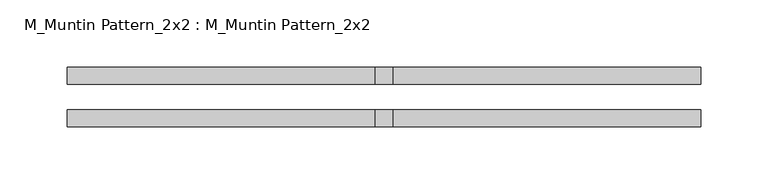
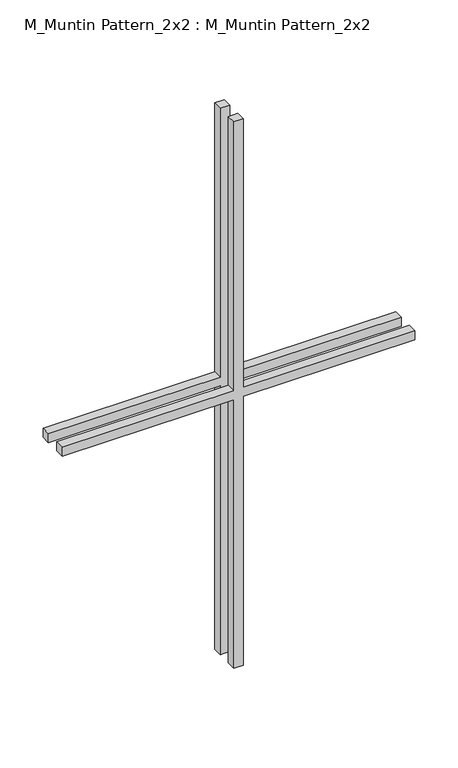
"""IFC4 building model written with IfcOpenShell, lengths in millimetres: proxy geometry, M_Muntin Pattern_2x2 : M_Muntin Pattern_2x2."""

from ifc_helpers import new_model, si_unit, frame, origin, place, context, project, spatial, polyline, outline, extrude, source, transform, mapped, element, save


def m_muntin_pattern_2x2_m_muntin_pattern_2x2_2357e71d(model_context):
    return source(origin(), model_context, "Body", "SweptSolid", [
        extrude(outline(polyline([(393.7, -6.35), (393.7, -236.5375), (381.0, -236.5375), (381.0, -6.35), (0.0, -6.35), (0.0, 6.35), (381.0, 6.35), (381.0, 236.5375), (393.7, 236.5375), (393.7, 6.35), (774.7, 6.35), (774.7, -6.35), (393.7, -6.35)])), frame((0.0, 9.525, 0.0), z_axis=(0.0, 1.0, 0.0), x_axis=(0.0, 0.0, 1.0)), (0.0, 0.0, 1.0), 12.7),
        extrude(outline(polyline([(393.7, -6.35), (393.7, -236.5375), (381.0, -236.5375), (381.0, -6.35), (0.0, -6.35), (0.0, 6.35), (381.0, 6.35), (381.0, 236.5375), (393.7, 236.5375), (393.7, 6.35), (774.7, 6.35), (774.7, -6.35), (393.7, -6.35)])), frame((0.0, -22.225, 0.0), z_axis=(0.0, 1.0, 0.0), x_axis=(0.0, 0.0, 1.0)), (0.0, 0.0, 1.0), 12.7),
    ])


if __name__ == "__main__":
    model = new_model("IFC4")
    model_context = context("Model", 3, world=origin())
    ifc_project = project(units=[si_unit("LENGTHUNIT", "METRE", prefix="MILLI")], contexts=[model_context])
    site = spatial("IfcSite", under=ifc_project)
    building = spatial("IfcBuilding", under=site)
    placement = place(None, origin())
    m_muntin_pattern_2x2_m_muntin_pattern_2x2_shape = m_muntin_pattern_2x2_m_muntin_pattern_2x2_2357e71d(model_context)
    element("IfcBuildingElementProxy", 1, Name="M_Muntin Pattern_2x2 : M_Muntin Pattern_2x2", ObjectType="M_Muntin Pattern_2x2 : M_Muntin Pattern_2x2", at=placement, inside=building, context=model_context, shape_type="MappedRepresentation", body=[
        mapped(m_muntin_pattern_2x2_m_muntin_pattern_2x2_shape, transform((0.0, 0.0, 0.0), x_axis=(1.0, 0.0, 0.0), y_axis=(0.0, 1.0, 0.0), z_axis=(0.0, 0.0, 1.0))),
    ])
    save(model, "model.ifc")

# Revit data of these elements
# Type "M_Muntin Pattern_2x2 : M_Muntin Pattern_2x2"
#   Width [instance default] = 3' - 11.24409"
#   Thickness = 0' - 0 1/2"
#   Height [instance default] = 3' - 11.24409"
#   Distance = 0' - 0 3/4"
#   Interior Material [instance default] = none
#   Exterior Material [instance default] = none
#   Default Elevation = 0
# Element 1 (IfcBuildingElementProxy, "M_Muntin Pattern_2x2 : M_Muntin Pattern_2x2")
#   Width = 1' - 6 5/8"
#   Height = 2' - 6 1/2"
#   Interior Material = Wood - Stained
#   Exterior Material = Clad - White
#   Materials on its faces: "Clad - White", "Wood - Stained"
# Materials
#   "Clad - White": class "Wood", colour RGB 242 242 238, transparency 0, Cost = 0
#   "Wood - Stained": class "Wood", colour RGB 224 178 126, transparency 0, Cost = 0
